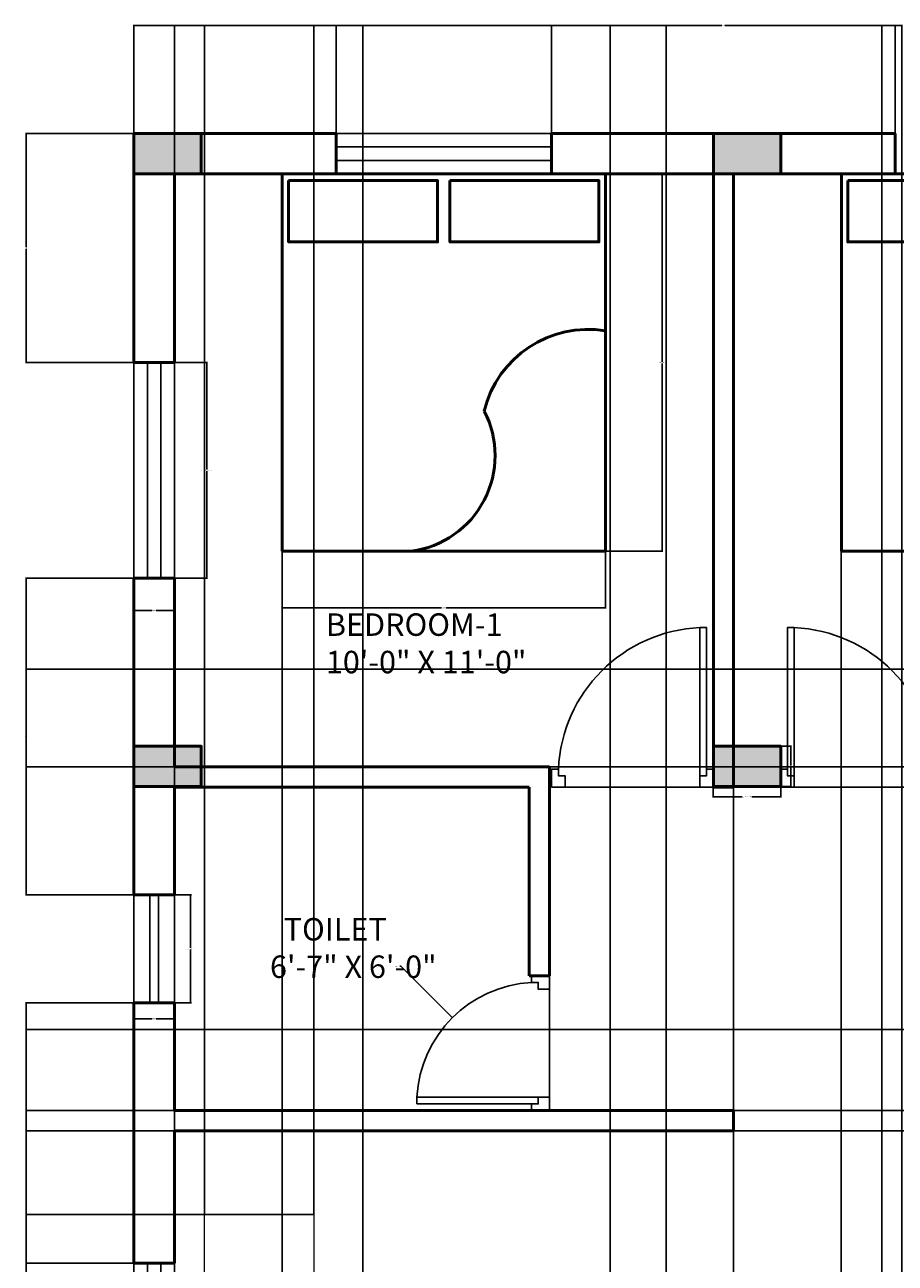
# Model space of a CAD drawing. Units: inches. Extents: x 2480 to 2840, y 795 to 1323.
# Tile 3 of 4: x 2480 to 2673, y 1047 to 1323. Entities that reach past the tile are written whole.
import ezdxf

# ---------------------------------------------------------------- set-up
doc = ezdxf.new("R2010")
doc.units = ezdxf.units.IN
for name, color, linetype, lineweight in [('A-ANNO-DIMS', 2, 'Continuous', 18), ('A-AREA-IDEN', 7, 'Continuous', 25), ('COLUMN', 240, 'Continuous', 50), ('door', 140, 'Continuous', 25), ('Furniture', 9, 'Continuous', 18), ('ventilator', 32, 'Continuous', 25), ('wall', 7, 'Continuous', 50), ('window', 201, 'Continuous', 25)]:
    doc.layers.add(name, color=color, linetype=linetype, lineweight=lineweight)
doc.styles.get("Standard").update_dxf_attribs({"font": 'arial.ttf'})
doc.dimstyles.get("Standard").update_dxf_attribs({"dimtxt": 0.18, "dimasz": 0.18, "dimexe": 0.18, "dimexo": 0.0625, "dimgap": 0.09, "dimtad": 0, "dimtih": 1, "dimtoh": 1, "dimdec": 4, "dimzin": 0, "dimdsep": 46, "dimtxsty": 'Standard', "dimcen": 0.09, "dimadec": 0, "dimazin": 0, "dimtfac": 1, "dimtdec": 4, "dimtofl": 0, "dimtmove": 0, "dimatfit": 3, "dimfxl": 1, "dimtolj": 1, "dimtzin": 0, "dimarcsym": 0})

# ---------------------------------------------------------------- blocks, each defined once
blk = doc.blocks.new('d1')
at = {"layer": 'door'}
blk.add_line((3049.73, 1052.02), (3085.73, 1052.02), dxfattribs=at)
blk.add_lwpolyline([(3051.23, 1054.52), (3052.73, 1054.52), (3052.73, 1087.52), (3051.23, 1087.52)], close=True, dxfattribs=at)
for points in [[(3052.73, 1052.02), (3049.73, 1052.02), (3049.73, 1056.02), (3051.23, 1056.02), (3051.23, 1054.52), (3052.73, 1054.52), (3052.73, 1052.02)], [(3082.73, 1052.02), (3085.73, 1052.02), (3085.73, 1056.02), (3084.23, 1056.02), (3084.23, 1054.52), (3082.73, 1054.52), (3082.73, 1052.02)]]:
    blk.add_lwpolyline(points, dxfattribs=at)
blk.add_arc((3051.23, 1054.52), 33.03, 2.6026, 87.3974, dxfattribs=at)
blk = doc.blocks.new('d2')
at = {"layer": 'door'}
blk.add_line((3049.73, 993.24), (3079.73, 993.24), dxfattribs=at)
blk.add_lwpolyline([(3051.23, 995.74), (3052.73, 995.74), (3052.73, 1022.74), (3051.23, 1022.74)], close=True, dxfattribs=at)
for points in [[(3052.73, 993.24), (3049.73, 993.24), (3049.73, 997.24), (3051.23, 997.24), (3051.23, 995.74), (3052.73, 995.74), (3052.73, 993.24)], [(3076.73, 993.24), (3079.73, 993.24), (3079.73, 997.24), (3078.23, 997.24), (3078.23, 995.74), (3076.73, 995.74), (3076.73, 993.24)]]:
    blk.add_lwpolyline(points, dxfattribs=at)
blk.add_arc((3051.23, 995.74), 27.04, 3.1798, 86.8202, dxfattribs=at)
blk = doc.blocks.new('w1')
at = {"layer": 'window'}
for p, q in [((2922.2, 1100.57), (2922.2, 1052.57)), ((2925.2, 1100.57), (2925.2, 1052.57))]:
    blk.add_line(p, q, dxfattribs=at)
blk.add_lwpolyline([(2919.2, 1052.57), (2928.2, 1052.57), (2928.2, 1100.57), (2919.2, 1100.57)], close=True, dxfattribs=at)
blk = doc.blocks.new('v')
at = {"layer": 'ventilator'}
for p, q in [((2939.68, 1237.47), (2939.68, 1213.47)), ((2941.68, 1237.47), (2941.68, 1213.47))]:
    blk.add_line(p, q, dxfattribs=at)
blk.add_lwpolyline([(2936.18, 1213.47), (2945.18, 1213.47), (2945.18, 1237.47), (2936.18, 1237.47)], close=True, dxfattribs=at)
blk = doc.blocks.new('BED')
at = {"layer": 'wall'}
for points in [[(3037.98, 1220.47), (3109.98, 1220.47), (3109.98, 1304.47), (3037.98, 1304.47)], [(3039.4, 1302.95), (3072.6, 1302.95), (3072.6, 1289.33), (3039.4, 1289.33)], [(3075.32, 1302.95), (3108.52, 1302.95), (3108.52, 1289.33), (3075.32, 1289.33)]]:
    blk.add_lwpolyline(points, close=True, dxfattribs=at)
for centre, radius, start, end in [((3106.11, 1246.04), 23.81, 80.6483, 166.366), ((3063.91, 1241.76), 21.48, 277.4854, 27.4236)]:
    blk.add_arc(centre, radius, start, end, dxfattribs=at)
blk = doc.blocks.new('C')
at = {"layer": 'COLUMN'}
h = blk.add_hatch(color=256, dxfattribs=at)
h.dxf.hatch_style = 1
h.paths.add_polyline_path([(3016.24, 1218.72), (3031.24, 1218.72), (3031.24, 1227.72), (3016.24, 1227.72)])
blk.add_lwpolyline([(3016.24, 1218.72), (3031.24, 1218.72), (3031.24, 1227.72), (3016.24, 1227.72)], close=True, dxfattribs=at)
blk = doc.blocks.new('*D10')
at = {"layer": 'A-ANNO-DIMS', "color": 0, "lineweight": -2, "transparency": 16777216}
for p, q in [((2632.95, 1153.27), (2632.95, 1150.9)), ((2647.95, 1153.27), (2647.95, 1150.9)), ((2633.13, 1151.08), (2639.35, 1151.08)), ((2647.77, 1151.08), (2641.56, 1151.08))]:
    blk.add_line(p, q, dxfattribs=at)
at = {"layer": 'A-ANNO-DIMS', "color": 0, "transparency": 16777216}
for points in [[(2633.13, 1151.11), (2633.13, 1151.05), (2632.95, 1151.08)], [(2647.77, 1151.11), (2647.77, 1151.05), (2647.95, 1151.08)]]:
    blk.add_solid(points, dxfattribs=at)
at = {"layer": 'Defpoints', "color": 0, "transparency": 16777216}
for p in [(2632.95, 1153.33), (2647.95, 1153.33), (2647.95, 1151.08)]:
    blk.add_point(p, dxfattribs=at)
at = {"layer": 'A-ANNO-DIMS', "color": 0, "transparency": 16777216, "insert": (2640.45, 1151.08), "char_height": 0.18, "attachment_point": 5}
blk.add_mtext('\\A1;COLUMN 15 TYP.', dxfattribs=at)
blk = doc.blocks.new('*D11')
at = {"layer": 'A-ANNO-DIMS', "color": 0, "lineweight": -2, "transparency": 16777216}
for p, q in [((2648.02, 1162.33), (2650.38, 1162.33)), ((2650.2, 1162.15), (2650.2, 1158.01)), ((2650.2, 1153.51), (2650.2, 1157.65)), ((2648.02, 1153.33), (2650.38, 1153.33))]:
    blk.add_line(p, q, dxfattribs=at)
at = {"layer": 'A-ANNO-DIMS', "color": 0, "transparency": 16777216}
for points in [[(2650.17, 1162.15), (2650.23, 1162.15), (2650.2, 1162.33)], [(2650.17, 1153.51), (2650.23, 1153.51), (2650.2, 1153.33)]]:
    blk.add_solid(points, dxfattribs=at)
at = {"layer": 'Defpoints', "color": 0, "transparency": 16777216}
for p in [(2647.95, 1162.33), (2650.2, 1162.33), (2647.95, 1153.33)]:
    blk.add_point(p, dxfattribs=at)
at = {"layer": 'A-ANNO-DIMS', "color": 0, "transparency": 16777216, "insert": (2650.2, 1157.83), "char_height": 0.18, "attachment_point": 5}
blk.add_mtext('\\A1;9 TYP.', dxfattribs=at)
blk = doc.blocks.new('*D12')
at = {"layer": 'A-ANNO-DIMS', "color": 0, "lineweight": -2, "transparency": 16777216}
for p, q in [((2513.02, 1247.74), (2520.33, 1247.74)), ((2520.15, 1247.56), (2520.15, 1223.92)), ((2520.15, 1199.92), (2520.15, 1223.56)), ((2513.02, 1199.74), (2520.33, 1199.74))]:
    blk.add_line(p, q, dxfattribs=at)
at = {"layer": 'A-ANNO-DIMS', "color": 0, "transparency": 16777216}
for points in [[(2520.12, 1247.56), (2520.18, 1247.56), (2520.15, 1247.74)], [(2520.12, 1199.92), (2520.18, 1199.92), (2520.15, 1199.74)]]:
    blk.add_solid(points, dxfattribs=at)
at = {"layer": 'Defpoints', "color": 0, "transparency": 16777216}
for p in [(2512.95, 1247.74), (2520.15, 1247.74), (2512.95, 1199.74)]:
    blk.add_point(p, dxfattribs=at)
at = {"layer": 'A-ANNO-DIMS', "color": 0, "transparency": 16777216, "insert": (2520.15, 1223.74), "char_height": 0.18, "attachment_point": 5}
blk.add_mtext('\\A1;WINDOW W1 48 TYP.', dxfattribs=at)
blk = doc.blocks.new('*D13')
at = {"layer": 'A-ANNO-DIMS', "color": 0, "lineweight": -2, "transparency": 16777216}
for p, q in [((2503.95, 1199.68), (2503.95, 1192.36)), ((2512.95, 1199.68), (2512.95, 1192.36)), ((2504.13, 1192.54), (2508, 1192.54)), ((2512.77, 1192.54), (2508.91, 1192.54))]:
    blk.add_line(p, q, dxfattribs=at)
at = {"layer": 'A-ANNO-DIMS', "color": 0, "transparency": 16777216}
for points in [[(2504.13, 1192.57), (2504.13, 1192.51), (2503.95, 1192.54)], [(2512.77, 1192.57), (2512.77, 1192.51), (2512.95, 1192.54)]]:
    blk.add_solid(points, dxfattribs=at)
at = {"layer": 'Defpoints', "color": 0, "transparency": 16777216}
for p in [(2503.95, 1199.74), (2512.95, 1199.74), (2512.95, 1192.54)]:
    blk.add_point(p, dxfattribs=at)
at = {"layer": 'A-ANNO-DIMS', "color": 0, "transparency": 16777216, "insert": (2508.45, 1192.54), "char_height": 0.18, "attachment_point": 5}
blk.add_mtext('\\A1;9 TYP.', dxfattribs=at)
blk = doc.blocks.new('*D16')
at = {"layer": 'A-ANNO-DIMS', "color": 0, "lineweight": -2, "transparency": 16777216}
for p, q in [((2513.02, 1129.24), (2516.73, 1129.24)), ((2516.55, 1129.06), (2516.55, 1117.42)), ((2516.55, 1105.42), (2516.55, 1117.06)), ((2513.02, 1105.24), (2516.73, 1105.24))]:
    blk.add_line(p, q, dxfattribs=at)
at = {"layer": 'A-ANNO-DIMS', "color": 0, "transparency": 16777216}
for points in [[(2516.52, 1129.06), (2516.58, 1129.06), (2516.55, 1129.24)], [(2516.52, 1105.42), (2516.58, 1105.42), (2516.55, 1105.24)]]:
    blk.add_solid(points, dxfattribs=at)
at = {"layer": 'Defpoints', "color": 0, "transparency": 16777216}
for p in [(2512.95, 1129.24), (2516.55, 1129.24), (2512.95, 1105.24)]:
    blk.add_point(p, dxfattribs=at)
at = {"layer": 'A-ANNO-DIMS', "color": 0, "transparency": 16777216, "insert": (2516.55, 1117.24), "char_height": 0.18, "attachment_point": 5}
blk.add_mtext('\\A1;VENT 24 TYP.', dxfattribs=at)
blk = doc.blocks.new('*D17')
at = {"layer": 'A-ANNO-DIMS', "color": 0, "lineweight": -2, "transparency": 16777216}
for p, q in [((2503.95, 1105.18), (2503.95, 1101.46)), ((2512.95, 1105.18), (2512.95, 1101.46)), ((2504.13, 1101.64), (2508, 1101.64)), ((2512.77, 1101.64), (2508.91, 1101.64))]:
    blk.add_line(p, q, dxfattribs=at)
at = {"layer": 'A-ANNO-DIMS', "color": 0, "transparency": 16777216}
for points in [[(2504.13, 1101.67), (2504.13, 1101.61), (2503.95, 1101.64)], [(2512.77, 1101.67), (2512.77, 1101.61), (2512.95, 1101.64)]]:
    blk.add_solid(points, dxfattribs=at)
at = {"layer": 'Defpoints', "color": 0, "transparency": 16777216}
for p in [(2503.95, 1105.24), (2512.95, 1105.24), (2512.95, 1101.64)]:
    blk.add_point(p, dxfattribs=at)
at = {"layer": 'A-ANNO-DIMS', "color": 0, "transparency": 16777216, "insert": (2508.45, 1101.64), "char_height": 0.18, "attachment_point": 5}
blk.add_mtext('\\A1;9 TYP.', dxfattribs=at)
blk = doc.blocks.new('*D24')
at = {"layer": 'A-ANNO-DIMS', "color": 0, "lineweight": -2, "transparency": 16777216}
for p, q in [((2609.02, 1289.74), (2621.73, 1289.74)), ((2621.55, 1289.56), (2621.55, 1247.92)), ((2621.55, 1205.92), (2621.55, 1247.56)), ((2609.02, 1205.74), (2621.73, 1205.74))]:
    blk.add_line(p, q, dxfattribs=at)
at = {"layer": 'A-ANNO-DIMS', "color": 0, "transparency": 16777216}
for points in [[(2621.52, 1289.56), (2621.58, 1289.56), (2621.55, 1289.74)], [(2621.52, 1205.92), (2621.58, 1205.92), (2621.55, 1205.74)]]:
    blk.add_solid(points, dxfattribs=at)
at = {"layer": 'Defpoints', "color": 0, "transparency": 16777216}
for p in [(2608.95, 1289.74), (2621.55, 1289.74), (2608.95, 1205.74)]:
    blk.add_point(p, dxfattribs=at)
at = {"layer": 'A-ANNO-DIMS', "color": 0, "transparency": 16777216, "insert": (2621.55, 1247.74), "char_height": 0.18, "attachment_point": 5}
blk.add_mtext('\\A1;BED 84 TYP.', dxfattribs=at)
blk = doc.blocks.new('*D25')
at = {"layer": 'A-ANNO-DIMS', "color": 0, "lineweight": -2, "transparency": 16777216}
for p, q in [((2536.95, 1205.68), (2536.95, 1192.96)), ((2608.95, 1205.68), (2608.95, 1192.96)), ((2537.13, 1193.14), (2572.43, 1193.14)), ((2608.77, 1193.14), (2573.48, 1193.14))]:
    blk.add_line(p, q, dxfattribs=at)
at = {"layer": 'A-ANNO-DIMS', "color": 0, "transparency": 16777216}
for points in [[(2537.13, 1193.17), (2537.13, 1193.11), (2536.95, 1193.14)], [(2608.77, 1193.17), (2608.77, 1193.11), (2608.95, 1193.14)]]:
    blk.add_solid(points, dxfattribs=at)
at = {"layer": 'Defpoints', "color": 0, "transparency": 16777216}
for p in [(2536.95, 1205.74), (2608.95, 1205.74), (2608.95, 1193.14)]:
    blk.add_point(p, dxfattribs=at)
at = {"layer": 'A-ANNO-DIMS', "color": 0, "transparency": 16777216, "insert": (2572.95, 1193.14), "char_height": 0.18, "attachment_point": 5}
blk.add_mtext('\\A1;72 TYP.', dxfattribs=at)
blk = doc.blocks.new('*D30')
at = {"layer": 'A-ANNO-DIMS', "color": 0, "lineweight": -2, "transparency": 16777216}
for p, q in [((2503.95, 1298.8), (2503.95, 1322.93)), ((2504.13, 1322.75), (2526.23, 1322.75)), ((2548.77, 1322.75), (2526.68, 1322.75)), ((2548.95, 1298.8), (2548.95, 1322.93))]:
    blk.add_line(p, q, dxfattribs=at)
at = {"layer": 'A-ANNO-DIMS', "color": 0, "transparency": 16777216}
for points in [[(2504.13, 1322.78), (2504.13, 1322.72), (2503.95, 1322.75)], [(2548.77, 1322.78), (2548.77, 1322.72), (2548.95, 1322.75)]]:
    blk.add_solid(points, dxfattribs=at)
at = {"layer": 'Defpoints', "color": 0, "transparency": 16777216}
for p in [(2548.95, 1322.75), (2503.95, 1298.74), (2548.95, 1298.74)]:
    blk.add_point(p, dxfattribs=at)
at = {"layer": 'A-ANNO-DIMS', "color": 0, "transparency": 16777216, "insert": (2526.45, 1322.75), "char_height": 0.18, "attachment_point": 5}
blk.add_mtext('\\A1;45', dxfattribs=at)
blk = doc.blocks.new('*D31')
at = {"layer": 'A-ANNO-DIMS', "color": 0, "lineweight": -2, "transparency": 16777216}
for p, q in [((2596.95, 1298.8), (2596.95, 1322.93)), ((2597.13, 1322.75), (2634.88, 1322.75)), ((2673.27, 1322.75), (2635.53, 1322.75)), ((2673.45, 1298.8), (2673.45, 1322.93))]:
    blk.add_line(p, q, dxfattribs=at)
at = {"layer": 'A-ANNO-DIMS', "color": 0, "transparency": 16777216}
for points in [[(2597.13, 1322.78), (2597.13, 1322.72), (2596.95, 1322.75)], [(2673.27, 1322.78), (2673.27, 1322.72), (2673.45, 1322.75)]]:
    blk.add_solid(points, dxfattribs=at)
at = {"layer": 'Defpoints', "color": 0, "transparency": 16777216}
for p in [(2673.45, 1322.75), (2596.95, 1298.74), (2673.45, 1298.74)]:
    blk.add_point(p, dxfattribs=at)
at = {"layer": 'A-ANNO-DIMS', "color": 0, "transparency": 16777216, "insert": (2635.2, 1322.75), "char_height": 0.18, "attachment_point": 5}
blk.add_mtext('\\A1;76.5', dxfattribs=at)
blk = doc.blocks.new('*D33')
at = {"layer": 'A-ANNO-DIMS', "color": 0, "lineweight": -2, "transparency": 16777216}
for p, q in [((2503.89, 1298.74), (2479.77, 1298.74)), ((2479.95, 1298.56), (2479.95, 1273.42)), ((2479.95, 1247.92), (2479.95, 1273.06)), ((2503.89, 1247.74), (2479.77, 1247.74))]:
    blk.add_line(p, q, dxfattribs=at)
at = {"layer": 'A-ANNO-DIMS', "color": 0, "transparency": 16777216}
for points in [[(2479.92, 1298.56), (2479.98, 1298.56), (2479.95, 1298.74)], [(2479.92, 1247.92), (2479.98, 1247.92), (2479.95, 1247.74)]]:
    blk.add_solid(points, dxfattribs=at)
at = {"layer": 'Defpoints', "color": 0, "transparency": 16777216}
for p in [(2503.95, 1298.74), (2479.95, 1247.74), (2503.95, 1247.74)]:
    blk.add_point(p, dxfattribs=at)
at = {"layer": 'A-ANNO-DIMS', "color": 0, "transparency": 16777216, "insert": (2479.95, 1273.24), "char_height": 0.18, "attachment_point": 5}
blk.add_mtext('\\A1;51', dxfattribs=at)
blk = doc.blocks.new('*D34')
at = {"layer": 'A-ANNO-DIMS', "color": 0, "lineweight": -2, "transparency": 16777216}
for p, q in [((2503.89, 1199.74), (2479.77, 1199.74)), ((2479.95, 1199.56), (2479.95, 1164.67)), ((2479.95, 1129.42), (2479.95, 1164.31)), ((2503.89, 1129.24), (2479.77, 1129.24))]:
    blk.add_line(p, q, dxfattribs=at)
at = {"layer": 'A-ANNO-DIMS', "color": 0, "transparency": 16777216}
for points in [[(2479.92, 1199.56), (2479.98, 1199.56), (2479.95, 1199.74)], [(2479.92, 1129.42), (2479.98, 1129.42), (2479.95, 1129.24)]]:
    blk.add_solid(points, dxfattribs=at)
at = {"layer": 'Defpoints', "color": 0, "transparency": 16777216}
for p in [(2503.95, 1199.74), (2479.95, 1129.24), (2503.95, 1129.24)]:
    blk.add_point(p, dxfattribs=at)
at = {"layer": 'A-ANNO-DIMS', "color": 0, "transparency": 16777216, "insert": (2479.95, 1164.49), "char_height": 0.18, "attachment_point": 5}
blk.add_mtext('\\A1;70.5', dxfattribs=at)
blk = doc.blocks.new('*D35')
at = {"layer": 'A-ANNO-DIMS', "color": 0, "lineweight": -2, "transparency": 16777216}
for p, q in [((2503.89, 1105.24), (2479.77, 1105.24)), ((2479.95, 1105.06), (2479.95, 1076.42)), ((2479.95, 1047.42), (2479.95, 1076.06)), ((2503.89, 1047.24), (2479.77, 1047.24))]:
    blk.add_line(p, q, dxfattribs=at)
at = {"layer": 'A-ANNO-DIMS', "color": 0, "transparency": 16777216}
for points in [[(2479.92, 1105.06), (2479.98, 1105.06), (2479.95, 1105.24)], [(2479.92, 1047.42), (2479.98, 1047.42), (2479.95, 1047.24)]]:
    blk.add_solid(points, dxfattribs=at)
at = {"layer": 'Defpoints', "color": 0, "transparency": 16777216}
for p in [(2503.95, 1105.24), (2479.95, 1047.24), (2503.95, 1047.24)]:
    blk.add_point(p, dxfattribs=at)
at = {"layer": 'A-ANNO-DIMS', "color": 0, "transparency": 16777216, "insert": (2479.95, 1076.24), "char_height": 0.18, "attachment_point": 5}
blk.add_mtext('\\A1;58', dxfattribs=at)
blk = doc.blocks.new('*D39')
at = {"layer": 'A-ANNO-DIMS', "color": 0, "lineweight": -2, "transparency": 16777216}
for p, q in [((2806.89, 1099.24), (2479.77, 1099.24)), ((2479.95, 1099.06), (2479.95, 1090.42)), ((2479.95, 1081.42), (2479.95, 1090.06)), ((2806.89, 1081.24), (2479.77, 1081.24))]:
    blk.add_line(p, q, dxfattribs=at)
at = {"layer": 'A-ANNO-DIMS', "color": 0, "transparency": 16777216}
for points in [[(2479.92, 1099.06), (2479.98, 1099.06), (2479.95, 1099.24)], [(2479.92, 1081.42), (2479.98, 1081.42), (2479.95, 1081.24)]]:
    blk.add_solid(points, dxfattribs=at)
at = {"layer": 'Defpoints', "color": 0, "transparency": 16777216}
for p in [(2479.95, 1099.24), (2806.95, 1099.24), (2806.95, 1081.24)]:
    blk.add_point(p, dxfattribs=at)
at = {"layer": 'A-ANNO-DIMS', "color": 0, "transparency": 16777216, "insert": (2479.95, 1090.24), "char_height": 0.18, "attachment_point": 5}
blk.add_mtext('\\A1;18', dxfattribs=at)
blk = doc.blocks.new('*D40')
at = {"layer": 'A-ANNO-DIMS', "color": 0, "lineweight": -2, "transparency": 16777216}
for p, q in [((2806.89, 1179.49), (2479.77, 1179.49)), ((2479.95, 1179.31), (2479.95, 1168.8)), ((2479.95, 1157.92), (2479.95, 1168.43)), ((2806.89, 1157.74), (2479.77, 1157.74))]:
    blk.add_line(p, q, dxfattribs=at)
at = {"layer": 'A-ANNO-DIMS', "color": 0, "transparency": 16777216}
for points in [[(2479.92, 1179.31), (2479.98, 1179.31), (2479.95, 1179.49)], [(2479.92, 1157.92), (2479.98, 1157.92), (2479.95, 1157.74)]]:
    blk.add_solid(points, dxfattribs=at)
at = {"layer": 'Defpoints', "color": 0, "transparency": 16777216}
for p in [(2479.95, 1179.49), (2806.95, 1179.49), (2806.95, 1157.74)]:
    blk.add_point(p, dxfattribs=at)
at = {"layer": 'A-ANNO-DIMS', "color": 0, "transparency": 16777216, "insert": (2479.95, 1168.62), "char_height": 0.18, "attachment_point": 5}
blk.add_mtext('\\A1;21.75', dxfattribs=at)
blk = doc.blocks.new('*D42')
at = {"layer": 'A-ANNO-DIMS', "color": 0, "lineweight": -2, "transparency": 16777216}
for p, q in [((2512.95, 969.8), (2512.95, 1322.93)), ((2513.13, 1322.75), (2567.32, 1322.75)), ((2622.27, 1322.75), (2568.09, 1322.75)), ((2622.45, 969.8), (2622.45, 1322.93))]:
    blk.add_line(p, q, dxfattribs=at)
at = {"layer": 'A-ANNO-DIMS', "color": 0, "transparency": 16777216}
for points in [[(2513.13, 1322.78), (2513.13, 1322.72), (2512.95, 1322.75)], [(2622.27, 1322.78), (2622.27, 1322.72), (2622.45, 1322.75)]]:
    blk.add_solid(points, dxfattribs=at)
at = {"layer": 'Defpoints', "color": 0, "transparency": 16777216}
for p in [(2622.45, 1322.75), (2512.95, 969.74), (2622.45, 969.74)]:
    blk.add_point(p, dxfattribs=at)
at = {"layer": 'A-ANNO-DIMS', "color": 0, "transparency": 16777216, "insert": (2567.7, 1322.75), "char_height": 0.18, "attachment_point": 5}
blk.add_mtext('\\A1;109.5', dxfattribs=at)
blk = doc.blocks.new('*D44')
at = {"layer": 'A-ANNO-DIMS', "color": 0, "lineweight": -2, "transparency": 16777216}
for p, q in [((2706.39, 1076.74), (2479.77, 1076.74)), ((2479.95, 1076.56), (2479.95, 1023.42)), ((2479.95, 969.92), (2479.95, 1023.06)), ((2710.89, 969.74), (2479.77, 969.74))]:
    blk.add_line(p, q, dxfattribs=at)
at = {"layer": 'A-ANNO-DIMS', "color": 0, "transparency": 16777216}
for points in [[(2479.92, 1076.56), (2479.98, 1076.56), (2479.95, 1076.74)], [(2479.92, 969.92), (2479.98, 969.92), (2479.95, 969.74)]]:
    blk.add_solid(points, dxfattribs=at)
at = {"layer": 'Defpoints', "color": 0, "transparency": 16777216}
for p in [(2479.95, 1076.74), (2706.45, 1076.74), (2710.95, 969.74)]:
    blk.add_point(p, dxfattribs=at)
at = {"layer": 'A-ANNO-DIMS', "color": 0, "transparency": 16777216, "insert": (2479.95, 1023.24), "char_height": 0.18, "attachment_point": 5}
blk.add_mtext('\\A1;107', dxfattribs=at)
blk = doc.blocks.new('*D45')
at = {"layer": 'A-ANNO-DIMS', "color": 0, "lineweight": -2, "transparency": 16777216}
for p, q in [((2512.95, 923.3), (2512.95, 1322.93)), ((2513.13, 1322.75), (2533.73, 1322.75)), ((2554.77, 1322.75), (2534.18, 1322.75)), ((2554.95, 923.3), (2554.95, 1322.93))]:
    blk.add_line(p, q, dxfattribs=at)
at = {"layer": 'A-ANNO-DIMS', "color": 0, "transparency": 16777216}
for points in [[(2513.13, 1322.78), (2513.13, 1322.72), (2512.95, 1322.75)], [(2554.77, 1322.78), (2554.77, 1322.72), (2554.95, 1322.75)]]:
    blk.add_solid(points, dxfattribs=at)
at = {"layer": 'Defpoints', "color": 0, "transparency": 16777216}
for p in [(2554.95, 1322.75), (2512.95, 923.24), (2554.95, 923.24)]:
    blk.add_point(p, dxfattribs=at)
at = {"layer": 'A-ANNO-DIMS', "color": 0, "transparency": 16777216, "insert": (2533.95, 1322.75), "char_height": 0.18, "attachment_point": 5}
blk.add_mtext('\\A1;42', dxfattribs=at)
blk = doc.blocks.new('*D47')
at = {"layer": 'A-ANNO-DIMS', "color": 0, "lineweight": -2, "transparency": 16777216}
for p, q in [((2554.95, 845.3), (2554.95, 1322.93)), ((2555.13, 1322.75), (2582.23, 1322.75)), ((2609.77, 1322.75), (2582.67, 1322.75)), ((2609.95, 845.3), (2609.95, 1322.93))]:
    blk.add_line(p, q, dxfattribs=at)
at = {"layer": 'A-ANNO-DIMS', "color": 0, "transparency": 16777216}
for points in [[(2555.13, 1322.78), (2555.13, 1322.72), (2554.95, 1322.75)], [(2609.77, 1322.78), (2609.77, 1322.72), (2609.95, 1322.75)]]:
    blk.add_solid(points, dxfattribs=at)
at = {"layer": 'Defpoints', "color": 0, "transparency": 16777216}
for p in [(2609.95, 1322.75), (2554.95, 845.24), (2609.95, 845.24)]:
    blk.add_point(p, dxfattribs=at)
at = {"layer": 'A-ANNO-DIMS', "color": 0, "transparency": 16777216, "insert": (2582.45, 1322.75), "char_height": 0.18, "attachment_point": 5}
blk.add_mtext('\\A1;55', dxfattribs=at)
blk = doc.blocks.new('*D50')
at = {"layer": 'A-ANNO-DIMS', "color": 0, "lineweight": -2, "transparency": 16777216}
for p, q in [((2637.45, 1076.68), (2637.45, 794.56)), ((2706.45, 1076.68), (2706.45, 794.56)), ((2637.63, 794.74), (2671.73, 794.74)), ((2706.27, 794.74), (2672.17, 794.74))]:
    blk.add_line(p, q, dxfattribs=at)
at = {"layer": 'A-ANNO-DIMS', "color": 0, "transparency": 16777216}
for points in [[(2637.63, 794.77), (2637.63, 794.71), (2637.45, 794.74)], [(2706.27, 794.77), (2706.27, 794.71), (2706.45, 794.74)]]:
    blk.add_solid(points, dxfattribs=at)
at = {"layer": 'Defpoints', "color": 0, "transparency": 16777216}
for p in [(2637.45, 1076.74), (2706.45, 1076.74), (2706.45, 794.74)]:
    blk.add_point(p, dxfattribs=at)
at = {"layer": 'A-ANNO-DIMS', "color": 0, "transparency": 16777216, "insert": (2671.95, 794.74), "char_height": 0.18, "attachment_point": 5}
blk.add_mtext('\\A1;69', dxfattribs=at)
blk = doc.blocks.new('*D52')
at = {"layer": 'A-ANNO-DIMS', "color": 0, "lineweight": -2, "transparency": 16777216}
for p, q in [((2670.45, 818.8), (2670.45, 1322.93)), ((2670.63, 1322.75), (2672.45, 1322.75)), ((2674.77, 1322.75), (2672.96, 1322.75)), ((2674.95, 827.8), (2674.95, 1322.93))]:
    blk.add_line(p, q, dxfattribs=at)
at = {"layer": 'A-ANNO-DIMS', "color": 0, "transparency": 16777216}
for points in [[(2670.63, 1322.78), (2670.63, 1322.72), (2670.45, 1322.75)], [(2674.77, 1322.78), (2674.77, 1322.72), (2674.95, 1322.75)]]:
    blk.add_solid(points, dxfattribs=at)
at = {"layer": 'Defpoints', "color": 0, "transparency": 16777216}
for p in [(2674.95, 1322.75), (2674.95, 827.74), (2670.45, 818.74)]:
    blk.add_point(p, dxfattribs=at)
at = {"layer": 'A-ANNO-DIMS', "color": 0, "transparency": 16777216, "insert": (2672.7, 1322.75), "char_height": 0.18, "attachment_point": 5}
blk.add_mtext('\\A1;4.5', dxfattribs=at)
blk = doc.blocks.new('*D54')
at = {"layer": 'A-ANNO-DIMS', "color": 0, "lineweight": -2, "transparency": 16777216}
for p, q in [((2519.64, 1058.13), (2519.64, 1322.93)), ((2519.82, 1322.75), (2531.36, 1322.75)), ((2543.82, 1322.75), (2532.29, 1322.75)), ((2544, 1058.13), (2544, 1322.93))]:
    blk.add_line(p, q, dxfattribs=at)
at = {"layer": 'A-ANNO-DIMS', "color": 0, "transparency": 16777216}
for points in [[(2519.82, 1322.78), (2519.82, 1322.72), (2519.64, 1322.75)], [(2543.82, 1322.78), (2543.82, 1322.72), (2544, 1322.75)]]:
    blk.add_solid(points, dxfattribs=at)
at = {"layer": 'Defpoints', "color": 0, "transparency": 16777216}
for p in [(2544, 1322.75), (2519.64, 1058.07), (2544, 1058.07)]:
    blk.add_point(p, dxfattribs=at)
at = {"layer": 'A-ANNO-DIMS', "color": 0, "transparency": 16777216, "insert": (2531.82, 1322.75), "char_height": 0.18, "attachment_point": 5}
blk.add_mtext('\\A1;24.364', dxfattribs=at)
blk = doc.blocks.new('*D55')
at = {"layer": 'A-ANNO-DIMS', "color": 0, "lineweight": -2, "transparency": 16777216}
for p, q in [((2543.94, 1058.07), (2479.77, 1058.07)), ((2479.95, 1057.89), (2479.95, 1020.58)), ((2479.95, 982.91), (2479.95, 1020.21)), ((2543.94, 982.73), (2479.77, 982.73))]:
    blk.add_line(p, q, dxfattribs=at)
at = {"layer": 'A-ANNO-DIMS', "color": 0, "transparency": 16777216}
for points in [[(2479.92, 1057.89), (2479.98, 1057.89), (2479.95, 1058.07)], [(2479.92, 982.91), (2479.98, 982.91), (2479.95, 982.73)]]:
    blk.add_solid(points, dxfattribs=at)
at = {"layer": 'Defpoints', "color": 0, "transparency": 16777216}
for p in [(2479.95, 1058.07), (2544, 1058.07), (2544, 982.73)]:
    blk.add_point(p, dxfattribs=at)
at = {"layer": 'A-ANNO-DIMS', "color": 0, "transparency": 16777216, "insert": (2479.95, 1020.4), "char_height": 0.18, "attachment_point": 5}
blk.add_mtext('\\A1;75.34', dxfattribs=at)
blk = doc.blocks.new('*D65')
at = {"layer": 'A-ANNO-DIMS', "color": 0, "lineweight": -2, "transparency": 16777216}
for p, q in [((2512.95, 1289.68), (2512.95, 794.56)), ((2536.95, 1289.68), (2536.95, 794.56)), ((2513.13, 794.74), (2524.73, 794.74)), ((2536.77, 794.74), (2525.17, 794.74))]:
    blk.add_line(p, q, dxfattribs=at)
at = {"layer": 'A-ANNO-DIMS', "color": 0, "transparency": 16777216}
for points in [[(2513.13, 794.77), (2513.13, 794.71), (2512.95, 794.74)], [(2536.77, 794.77), (2536.77, 794.71), (2536.95, 794.74)]]:
    blk.add_solid(points, dxfattribs=at)
at = {"layer": 'Defpoints', "color": 0, "transparency": 16777216}
for p in [(2512.95, 1289.74), (2536.95, 1289.74), (2536.95, 794.74)]:
    blk.add_point(p, dxfattribs=at)
at = {"layer": 'A-ANNO-DIMS', "color": 0, "transparency": 16777216, "insert": (2524.95, 794.74), "char_height": 0.18, "attachment_point": 5}
blk.add_mtext('\\A1;24', dxfattribs=at)
blk = doc.blocks.new('*D66')
at = {"layer": 'A-ANNO-DIMS', "color": 0, "lineweight": -2, "transparency": 16777216}
for p, q in [((2637.45, 1289.68), (2637.45, 794.56)), ((2661.45, 1289.68), (2661.45, 794.56)), ((2637.63, 794.74), (2649.23, 794.74)), ((2661.27, 794.74), (2649.67, 794.74))]:
    blk.add_line(p, q, dxfattribs=at)
at = {"layer": 'A-ANNO-DIMS', "color": 0, "transparency": 16777216}
for points in [[(2637.63, 794.77), (2637.63, 794.71), (2637.45, 794.74)], [(2661.27, 794.77), (2661.27, 794.71), (2661.45, 794.74)]]:
    blk.add_solid(points, dxfattribs=at)
at = {"layer": 'Defpoints', "color": 0, "transparency": 16777216}
for p in [(2637.45, 1289.74), (2661.45, 1289.74), (2661.45, 794.74)]:
    blk.add_point(p, dxfattribs=at)
at = {"layer": 'A-ANNO-DIMS', "color": 0, "transparency": 16777216, "insert": (2649.45, 794.74), "char_height": 0.18, "attachment_point": 5}
blk.add_mtext('\\A1;24', dxfattribs=at)
blk = doc.blocks.new('*D70')
at = {"layer": 'A-ANNO-DIMS', "color": 0, "lineweight": -2, "transparency": 16777216}
for p, q in [((2563.18, 1113.34), (2563.36, 1113.34)), ((2563.36, 1113.34), (2574.7, 1101.99)), ((2593.86, 1082.74), (2594.04, 1082.74)), ((2593.95, 1082.65), (2593.95, 1082.83))]:
    blk.add_line(p, q, dxfattribs=at)
at = {"layer": 'A-ANNO-DIMS', "color": 0, "transparency": 16777216}
blk.add_solid([(2574.73, 1102.01), (2574.68, 1101.97), (2574.83, 1101.86)], dxfattribs=at)
at = {"layer": 'Defpoints', "color": 0, "transparency": 16777216}
for p in [(2574.83, 1101.86), (2593.95, 1082.74)]:
    blk.add_point(p, dxfattribs=at)
at = {"layer": 'A-ANNO-DIMS', "color": 0, "transparency": 16777216, "insert": (2562.51, 1113.34), "char_height": 0.18, "attachment_point": 5}
blk.add_mtext('\\A1;3X R27.04', dxfattribs=at)

msp = doc.modelspace()

# ---------------------------------------------------------------- linework, layer by layer
at = {"layer": 'Furniture'}
msp.add_lwpolyline([(2519.6396, 1058.0677), (2544.0036, 1058.0677), (2544.0036, 982.726), (2519.6396, 982.726)], close=True, dxfattribs=at)
at = {"layer": 'wall'}
for p, q in [((2503.9535, 1298.7416), (2503.9535, 1247.7416)), ((2548.9535, 1298.7416), (2503.9535, 1298.7416)), ((2548.9535, 1289.7416), (2548.9535, 1298.7416)), ((2596.9535, 1289.7416), (2596.9535, 1298.7416)), ((2673.4535, 1298.7416), (2596.9535, 1298.7416)), ((2673.4535, 1289.7416), (2673.4535, 1298.7416)), ((2512.9535, 1289.7416), (2512.9535, 1247.7416)), ((2548.9535, 1289.7416), (2512.9535, 1289.7416)), ((2632.9535, 1289.7416), (2596.9535, 1289.7416)), ((2632.9535, 1289.7416), (2632.9535, 1153.2416)), ((2637.4535, 1289.7416), (2637.4535, 1153.2416)), ((2673.4535, 1289.7416), (2637.4535, 1289.7416)), ((2512.9535, 1247.7416), (2503.9535, 1247.7416)), ((2512.9535, 1199.7416), (2503.9535, 1199.7416)), ((2503.9535, 1199.7416), (2503.9535, 1129.2416)), ((2512.9535, 1199.7416), (2512.9535, 1157.7416)), ((2596.4535, 1157.7416), (2512.9535, 1157.7416)), ((2596.4535, 1157.7416), (2596.4535, 1111.2416)), ((2512.9535, 1153.2416), (2512.9535, 1129.2416)), ((2591.9535, 1153.2416), (2512.9535, 1153.2416)), ((2591.9535, 1153.2416), (2591.9535, 1111.2416)), ((2632.9535, 1153.2416), (2637.4535, 1153.2416)), ((2512.9535, 1129.2416), (2503.9535, 1129.2416)), ((2596.4535, 1111.2416), (2591.9535, 1111.2416)), ((2512.9535, 1105.2416), (2503.9535, 1105.2416)), ((2503.9535, 1105.2416), (2503.9535, 1047.2416)), ((2512.9535, 1105.2416), (2512.9535, 1081.2416)), ((2596.4535, 1081.2416), (2512.9535, 1081.2416)), ((2632.9535, 1081.2416), (2596.4535, 1081.2416)), ((2632.9535, 1081.2416), (2637.4535, 1081.2416)), ((2637.4535, 1081.2416), (2637.4535, 1076.7416)), ((2632.9535, 1076.7416), (2512.9535, 1076.7416)), ((2512.9535, 1076.7416), (2512.9535, 1047.2416)), ((2632.9535, 1076.7416), (2637.4535, 1076.7416)), ((2512.9535, 1047.2416), (2503.9535, 1047.2416))]:
    msp.add_line(p, q, dxfattribs=at)

# ---------------------------------------------------------------- block references
at = {"layer": 'COLUMN'}
for p in [(-512.2865, 71.0183), (-383.2865, 71.0183), (-512.2865, -65.3906), (-383.2865, -65.3906)]:
    msp.add_blockref('C', p, dxfattribs=at)
at = {"layer": 'door', "xscale": -1}
msp.add_blockref('d1', (5682.6859, 101.2216), dxfattribs=at)
at = {"layer": 'door'}
msp.add_blockref('d1', (-401.7789, 101.2216), dxfattribs=at)
at = {"layer": 'door', "rotation": 90}
msp.add_blockref('d2', (3589.697, -1968.4908), dxfattribs=at)
at = {"layer": 'Furniture'}
for p in [(-501.025, -14.7245), (-376.525, -14.7245)]:
    msp.add_blockref('BED', p, dxfattribs=at)
at = {"layer": 'ventilator'}
msp.add_blockref('v', (-432.2266, -108.2301), dxfattribs=at)
at = {"layer": 'window', "rotation": 90}
msp.add_blockref('w1', (3649.5221, -1629.4626), dxfattribs=at)
at = {"layer": 'window'}
for p in [(-415.2506, 147.173), (-415.2506, -53.327)]:
    msp.add_blockref('w1', p, dxfattribs=at)

# ---------------------------------------------------------------- texts
at = {"layer": 'A-AREA-IDEN', "char_height": 5, "attachment_point": 1}
for s, insert in [('BEDROOM-1\\P10\'-0" X 11\'-0"', (2546.6778, 1191.8999)), ('  TOILET\\P6\'-7" X 6\'-0"', (2534.2406, 1124.0771))]:
    msp.add_mtext_dynamic_manual_height_columns(s, width=47.7919, gutter_width=12.5, heights=[0], dxfattribs=dict(at, insert=insert))

# ---------------------------------------------------------------- dimensions: what is measured, and where the dimension line sits
at = {"layer": 'A-ANNO-DIMS'}
for base, p1, p2, override, picture, middle in [((2548.9535, 1322.7466), (2503.9535, 1298.7416), (2548.9535, 1298.7416), {"dimdec": 0, "dimlfac": 1, "dimrnd": 0, "dimzin": 0, "dimdsep": 46, "dimlunit": 2}, '*D30', (2526.4535, 1322.7466)), ((2622.4535, 1322.7466), (2512.9535, 969.7416), (2622.4535, 969.7416), {"dimdec": 1, "dimlfac": 1, "dimrnd": 0, "dimzin": 0, "dimdsep": 46, "dimlunit": 2}, '*D42', (2567.7035, 1322.7466)), ((2554.9535, 1322.7466), (2512.9535, 923.2416), (2554.9535, 923.2416), {"dimdec": 0, "dimlfac": 1, "dimrnd": 0, "dimzin": 0, "dimdsep": 46, "dimlunit": 2}, '*D45', (2533.9535, 1322.7466)), ((2544.0036, 1322.7466), (2519.6396, 1058.0677), (2544.0036, 1058.0677), {"dimdec": 3, "dimlfac": 1, "dimrnd": 0, "dimzin": 0, "dimdsep": 46, "dimlunit": 2}, '*D54', (2531.8216, 1322.7466)), ((2609.9535, 1322.7466), (2554.9535, 845.2416), (2609.9535, 845.2416), {"dimdec": 0, "dimlfac": 1, "dimrnd": 0, "dimzin": 0, "dimdsep": 46, "dimlunit": 2}, '*D47', (2582.4535, 1322.7466)), ((2673.4535, 1322.7466), (2596.9535, 1298.7416), (2673.4535, 1298.7416), {"dimdec": 1, "dimlfac": 1, "dimrnd": 0, "dimzin": 0, "dimdsep": 46, "dimlunit": 2}, '*D31', (2635.2035, 1322.7466)), ((2674.9535, 1322.7466), (2670.4535, 818.7416), (2674.9535, 827.7416), {"dimdec": 1, "dimlfac": 1, "dimrnd": 0, "dimzin": 0, "dimdsep": 46, "dimlunit": 2}, '*D52', (2672.7035, 1322.7466)), ((2536.9535, 794.7366), (2512.9535, 1289.7416), (2536.9535, 1289.7416), {"dimdec": 0, "dimlfac": 1, "dimrnd": 0, "dimzin": 0, "dimdsep": 46, "dimlunit": 2}, '*D65', (2524.9535, 794.7366)), ((2661.4535, 794.7366), (2637.4535, 1289.7416), (2661.4535, 1289.7416), {"dimdec": 0, "dimlfac": 1, "dimrnd": 0, "dimzin": 0, "dimdsep": 46, "dimlunit": 2}, '*D66', (2649.4535, 794.7366)), ((2706.4535, 794.7366), (2637.4535, 1076.7416), (2706.4535, 1076.7416), {"dimdec": 0, "dimlfac": 1, "dimrnd": 0, "dimzin": 0, "dimdsep": 46, "dimlunit": 2}, '*D50', (2671.9535, 794.7366))]:
    dim = msp.add_linear_dim(base=base, p1=p1, p2=p2, dimstyle='Standard', override=override, dxfattribs=at)
    dim.commit()
    dim.dimension.update_dxf_attribs({"geometry": picture, "text_midpoint": middle})
for base, p1, p2, override, picture, middle in [((2479.9485, 1247.7416), (2503.9535, 1298.7416), (2503.9535, 1247.7416), {"dimdec": 0, "dimlfac": 1, "dimrnd": 0, "dimzin": 0, "dimdsep": 46, "dimlunit": 2}, '*D33', (2479.9485, 1273.2416)), ((2479.9485, 1129.2416), (2503.9535, 1199.7416), (2503.9535, 1129.2416), {"dimdec": 1, "dimlfac": 1, "dimrnd": 0, "dimzin": 0, "dimdsep": 46, "dimlunit": 2}, '*D34', (2479.9485, 1164.4916)), ((2479.9485, 1179.4916), (2806.9535, 1157.7416), (2806.9535, 1179.4916), {"dimdec": 2, "dimlfac": 1, "dimrnd": 0, "dimzin": 0, "dimdsep": 46, "dimlunit": 2}, '*D40', (2479.9485, 1168.6166)), ((2479.9485, 1047.2416), (2503.9535, 1105.2416), (2503.9535, 1047.2416), {"dimdec": 0, "dimlfac": 1, "dimrnd": 0, "dimzin": 0, "dimdsep": 46, "dimlunit": 2}, '*D35', (2479.9485, 1076.2416)), ((2479.9485, 1099.2416), (2806.9535, 1081.2416), (2806.9535, 1099.2416), {"dimdec": 0, "dimlfac": 1, "dimrnd": 0, "dimzin": 0, "dimdsep": 46, "dimlunit": 2}, '*D39', (2479.9485, 1090.2416)), ((2479.9485, 1076.7416), (2710.9535, 969.7416), (2706.4535, 1076.7416), {"dimdec": 0, "dimlfac": 1, "dimrnd": 0, "dimzin": 0, "dimdsep": 46, "dimlunit": 2}, '*D44', (2479.9485, 1023.2416)), ((2479.9485, 1058.0677), (2544.0036, 982.726), (2544.0036, 1058.0677), {"dimdec": 2, "dimlfac": 1, "dimrnd": 0, "dimzin": 0, "dimdsep": 46, "dimlunit": 2}, '*D55', (2479.9485, 1020.3968))]:
    dim = msp.add_linear_dim(base=base, p1=p1, p2=p2, angle=90, dimstyle='Standard', override=override, dxfattribs=at)
    dim.commit()
    dim.dimension.update_dxf_attribs({"geometry": picture, "text_midpoint": middle})
for base, p1, p2, text, picture, middle in [((2621.5535, 1289.7416), (2608.9535, 1205.7416), (2608.9535, 1289.7416), 'BED <> TYP.', '*D24', (2621.5535, 1247.7416)), ((2520.1535, 1247.7416), (2512.9535, 1199.7416), (2512.9535, 1247.7416), 'WINDOW W1 <> TYP.', '*D12', (2520.1535, 1223.7416)), ((2650.2035, 1162.3327), (2647.9535, 1153.3327), (2647.9535, 1162.3327), '<> TYP.', '*D11', (2650.2035, 1157.8327)), ((2516.5535, 1129.2416), (2512.9535, 1105.2416), (2512.9535, 1129.2416), 'VENT <> TYP.', '*D16', (2516.5535, 1117.2416))]:
    dim = msp.add_linear_dim(base=base, p1=p1, p2=p2, angle=90, text=text, dimstyle='Standard', override={"dimdec": 0, "dimlfac": 1, "dimrnd": 0, "dimzin": 0, "dimdsep": 46, "dimlunit": 2}, dxfattribs=at)
    dim.commit()
    dim.dimension.update_dxf_attribs({"geometry": picture, "text_midpoint": middle})
for base, p1, p2, text, picture, middle in [((2608.9535, 1193.1416), (2536.9535, 1205.7416), (2608.9535, 1205.7416), '<> TYP.', '*D25', (2572.9535, 1193.1416)), ((2512.9535, 1192.5416), (2503.9535, 1199.7416), (2512.9535, 1199.7416), '<> TYP.', '*D13', (2508.4535, 1192.5416)), ((2647.9535, 1151.0827), (2632.9535, 1153.3327), (2647.9535, 1153.3327), 'COLUMN <> TYP.', '*D10', (2640.4535, 1151.0827)), ((2512.9535, 1101.6416), (2503.9535, 1105.2416), (2512.9535, 1105.2416), '<> TYP.', '*D17', (2508.4535, 1101.6416))]:
    dim = msp.add_linear_dim(base=base, p1=p1, p2=p2, text=text, dimstyle='Standard', override={"dimdec": 0, "dimlfac": 1, "dimrnd": 0, "dimzin": 0, "dimdsep": 46, "dimlunit": 2}, dxfattribs=at)
    dim.commit()
    dim.dimension.update_dxf_attribs({"geometry": picture, "text_midpoint": middle})
dim = msp.add_radius_dim(center=(2593.9535, 1082.7416), mpoint=(2574.8321, 1101.8629), text='3X <>', dimstyle='Standard', override={"dimdec": 2, "dimlfac": 1, "dimrnd": 0, "dimzin": 0, "dimdsep": 46, "dimlunit": 2}, dxfattribs=at)
dim.commit()
dim.dimension.update_dxf_attribs({"geometry": '*D70', "text_midpoint": (2562.5065, 1113.3356), "dimtype": 164})

doc.saveas('drawing.dxf')
